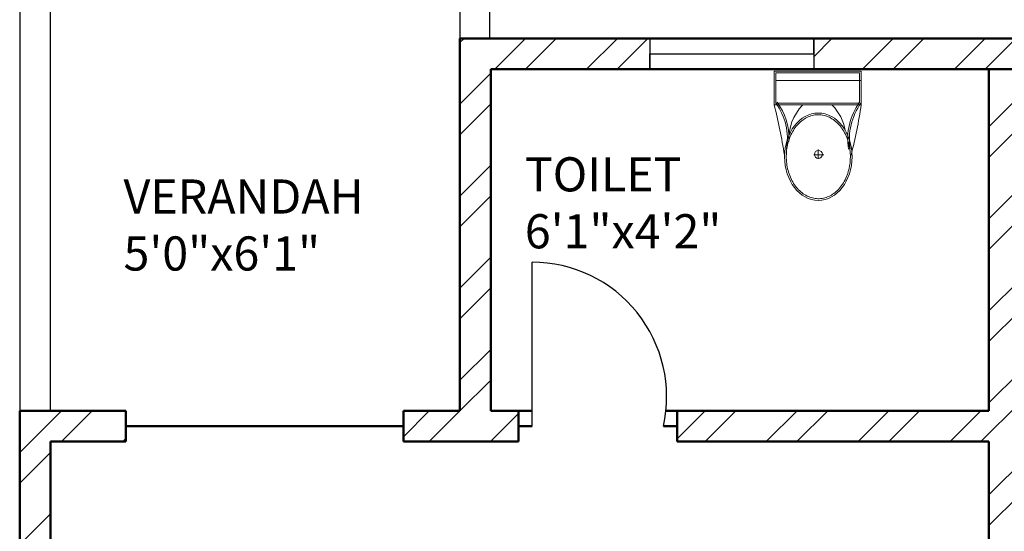
# Model space of a CAD drawing. Units: inches. Extents: x 1901 to 2863, y 888 to 2433.
# Tile 62 of 91: x 2025 to 2169, y 2202 to 2277. Entities that reach past the tile are written whole.
import ezdxf

# ---------------------------------------------------------------- set-up
doc = ezdxf.new("R2010")
doc.units = ezdxf.units.IN
for name, color, linetype, lineweight in [('A-AREA-IDEN', 7, 'Continuous', 18), ('A-DOOR', 4, 'Continuous', 25), ('A-FLOR-FIXT', 9, 'Continuous', 18), ('A-FLOR-HRAL', 41, 'Continuous', 25), ('A-GLAZ', 3, 'Continuous', 25), ('A-WALL', 7, 'Continuous', 50), ('A-WALL-PATT', 8, 'Continuous', 13)]:
    doc.layers.add(name, color=color, linetype=linetype, lineweight=lineweight)
doc.styles.get("Standard").update_dxf_attribs({"font": 'arial.ttf'})

# ---------------------------------------------------------------- blocks, each defined once
blk = doc.blocks.new('A$C31115884')
for p, q in [((283.1, 497.7), (223.4, 497.7)), ((257.5, 466.4), (257.5, 523.2)), ((0, 200), (0, 0)), ((520, 200), (0, 200)), ((10, 190), (10, 10)), ((510, 190), (10, 190)), ((510, 10), (510, 190)), ((520, 0), (520, 200)), ((510, 54.5), (0, 54.5)), ((10, 10), (510, 10)), ((0, 0), (520, 0))]:
    blk.add_line(p, q)
blk.add_circle((255.6, 496.4), 23.6)
for centre, radius, start, end in [((2777.7, -204.6), 2807, 165.4549, 171.71327), ((3237, 905), 2807, 188.28673, 194.5451), ((-294.5, 403.3), 364.7, 324.20913, 9.34987), ((-294.5, 403.3), 374.7, 324.20913, 9.34987), ((139.5, 406.2), 293.5, 315.84364, 2.65635), ((805.8, 403.3), 364.7, 170.65013, 215.79087), ((383.6, 406.2), 293.5, 190.27735, 224.15636), ((805.8, 403.3), 374.7, 179.20365, 215.79087)]:
    blk.add_arc(centre, radius, start, end)
blk.add_ellipse((256.2, 509.9), major_axis=(0, -260.7), ratio=0.772727)
blk.add_open_spline([(256.2, 259.2), (263.1, 259.2), (270, 259.7), (287.8, 262.3), (298.7, 265.1), (319.9, 273.1), (330.2, 278.4), (350.1, 291.1), (359.7, 298.7), (377.7, 315.9), (386.2, 325.5), (401.7, 346.6), (408.8, 358.1), (421.3, 382.5), (426.8, 395.5), (435.9, 422.4), (439.5, 436.4), (444.8, 465.1), (446.5, 479.7), (447.9, 509.2), (447.6, 524), (445, 553.3), (442.7, 567.8), (436.3, 596), (432.1, 609.7), (421.9, 636), (416, 648.6), (402.5, 672.1), (395, 683), (378.6, 703), (369.8, 712.1), (351.1, 728), (341.3, 734.8), (320.9, 746.2), (310.4, 750.7), (288.9, 757.3), (278, 759.4), (256, 761), (245, 760.6), (223.1, 757.2), (212.3, 754.3), (191.1, 746.1), (180.8, 740.7), (160.9, 727.8), (151.4, 720.1), (133.5, 702.7), (125.1, 693), (109.6, 671.7), (102.6, 660.2), (90.2, 635.7), (84.9, 622.7), (76, 595.6), (72.4, 581.6), (67.2, 552.9), (65.6, 538.2), (64.4, 508.8), (64.8, 494), (67.5, 464.7), (69.9, 450.2), (76.6, 422), (80.8, 408.3), (91.1, 382.2), (97.2, 369.7), (110.8, 346.3), (118.4, 335.4), (134.8, 315.6), (143.7, 306.7), (162.4, 290.9), (172.3, 284.2), (192.8, 273), (203.3, 268.6), (224.8, 262.2), (235.8, 260.2), (249.9, 259.3), (253, 259.2), (256.2, 259.2)], degree=3, knots=[0, 0, 0, 0, 0.110105, 0.110105, 0.285049, 0.285049, 0.459994, 0.459994, 0.634938, 0.634938, 0.809882, 0.809882, 0.984827, 0.984827, 1.159771, 1.159771, 1.334715, 1.334715, 1.50966, 1.50966, 1.684604, 1.684604, 1.859549, 1.859549, 2.034493, 2.034493, 2.209437, 2.209437, 2.384382, 2.384382, 2.559326, 2.559326, 2.73427, 2.73427, 2.909215, 2.909215, 3.084159, 3.084159, 3.259103, 3.259103, 3.434048, 3.434048, 3.608992, 3.608992, 3.783936, 3.783936, 3.958881, 3.958881, 4.133825, 4.133825, 4.30877, 4.30877, 4.483714, 4.483714, 4.658658, 4.658658, 4.833603, 4.833603, 5.008547, 5.008547, 5.183491, 5.183491, 5.358436, 5.358436, 5.53338, 5.53338, 5.708324, 5.708324, 5.883269, 5.883269, 6.058213, 6.058213, 6.233158, 6.233158, 6.283185, 6.283185, 6.283185, 6.283185])
blk = doc.blocks.new('WIN-24')
for p, q in [((0, 4.5), (0, 0)), ((24, 2.25), (24, 4.5)), ((24, 4.5), (24, 0)), ((0, 0), (0, 2.25)), ((0, 2.25), (24, 2.25))]:
    blk.add_line(p, q)
blk = doc.blocks.new('DOOR-20')
blk.add_line((0, -0.02), (0, 23.98))
blk.add_arc((0, 4.28), 19.71, 347.419, 90)

msp = doc.modelspace()

# ---------------------------------------------------------------- hatches: boundary and pattern name
at = {"layer": 'A-WALL-PATT'}
h = msp.add_hatch(dxfattribs=at)
h.set_pattern_fill('ANSI32', color=256)
h.paths.add_polyline_path([(2192.5, 2274.13), (2141.26, 2274.13), (2141.26, 2269.63), (2192.5, 2269.63)])
h.paths.add_polyline_path([(2259.93, 2274.13), (2216.5, 2274.13), (2216.5, 2269.63), (2255.43, 2269.63), (2255.43, 2214.63), (2250.81, 2214.63), (2250.81, 2210.13), (2259.93, 2210.13), (2259.93, 2215.13), (2271.76, 2215.13), (2271.76, 2217.38), (2271.76, 2219.63), (2259.93, 2219.63)])
h.paths.add_polyline_path([(2171.43, 2269.63), (2166.93, 2269.63), (2166.93, 2219.63), (2121.24, 2219.63), (2121.24, 2215.13), (2166.93, 2215.13), (2166.93, 2083.13), (2161.81, 2083.13), (2161.81, 2078.63), (2171.43, 2078.63), (2177, 2078.63), (2177, 2080.88), (2177, 2083.13), (2171.43, 2083.13), (2171.43, 2210.13), (2230.91, 2210.13), (2230.91, 2212.38), (2230.91, 2214.63), (2171.43, 2214.63)])
h.paths.add_polyline_path([(2117.26, 2274.13), (2089.43, 2274.13), (2089.43, 2219.63), (2081.14, 2219.63), (2081.14, 2215.13), (2089.43, 2215.13), (2098, 2215.13), (2098, 2217.38), (2098, 2219.63), (2093.93, 2219.63), (2093.93, 2269.63), (2117.26, 2269.63), (2117.26, 2271.88)])
h.paths.add_polyline_path([(2343.43, 2219.63), (2329.29, 2219.63), (2329.29, 2215.13), (2338.93, 2215.13), (2338.93, 2184.74), (2343.43, 2184.74)])
h.paths.add_polyline_path([(2338.93, 2083.13), (2329.29, 2083.13), (2208.97, 2083.13), (2208.97, 2078.63), (2338.93, 2078.63)])
h.paths.add_polyline_path([(2343.43, 2136.74), (2338.93, 2136.74), (2338.93, 1872.63), (2343.43, 1872.63)])
h.paths.add_polyline_path([(2343.43, 1863.63), (2397.68, 1863.63), (2397.68, 1821.63), (2384.14, 1821.63), (2384.14, 1812.63), (2418.33, 1812.63), (2418.33, 1817.13), (2418.33, 1821.63), (2406.68, 1821.63), (2406.68, 1863.63), (2459.5, 1863.63), (2459.5, 1821.63), (2447.14, 1821.63), (2447.14, 1812.63), (2459.5, 1812.63), (2468.5, 1812.63), (2468.5, 1872.63), (2394.43, 1872.63), (2334.43, 1872.63), (2334.43, 1812.63), (2343.43, 1812.63), (2353.25, 1812.63), (2353.25, 1821.63), (2343.43, 1821.63)])
h.paths.add_polyline_path([(2510.01, 1872.63), (2468.5, 1872.63), (2468.5, 1868.13), (2510.01, 1868.13)])
h.paths.add_polyline_path([(2514.01, 1817.13), (2468.5, 1817.13), (2468.5, 1812.63), (2482.11, 1812.63), (2482.11, 1800.61), (2486.61, 1800.61), (2486.61, 1812.63), (2514.01, 1812.63)])
h.paths.add_polyline_path([(2299.25, 1814.88), (2299.25, 1817.13), (2295.93, 1817.13), (2295.93, 1854.17), (2293.68, 1854.17), (2291.43, 1854.17), (2291.43, 1817.13), (2266.11, 1817.13), (2266.11, 1812.63), (2299.25, 1812.63)])
h.paths.add_polyline_path([(2218.11, 1817.13), (2206.46, 1817.13), (2171.43, 1817.13), (2171.43, 1949.13), (2190.1, 1949.13), (2190.1, 1953.63), (2163.47, 1953.63), (2163.47, 1949.13), (2166.93, 1949.13), (2166.93, 1817.13), (2114.3, 1817.13), (2114.3, 1812.63), (2218.11, 1812.63)])
h.paths.add_polyline_path([(2029.43, 1970.92), (2024.93, 1970.92), (2024.93, 1912.72), (2029.43, 1912.72)])
h.paths.add_polyline_path([(2132.3, 1953.63), (2113.93, 1953.63), (2113.93, 1975.89), (2111.68, 1975.89), (2109.43, 1975.89), (2109.43, 1953.63), (2029.43, 1953.63), (2029.43, 1949.13), (2132.3, 1949.13)])
h.paths.add_polyline_path([(2029.43, 1853.61), (2029.31, 1853.61), (2029.31, 1853.61), (2029.43, 1853.61), (2029.43, 1864.72), (2024.93, 1864.72), (2024.93, 1812.63), (2066.3, 1812.63), (2066.3, 1814.88), (2066.3, 1817.13), (2029.43, 1817.13)])
h.paths.add_polyline_path([(2122.93, 2010.09), (2120.68, 2010.09), (2118.43, 2010.09), (2118.43, 2006.13), (2029.43, 2006.13), (2029.43, 2001.63), (2109.43, 2001.63), (2109.43, 1998.04), (2113.93, 1998.04), (2113.93, 2001.63), (2122.93, 2001.63)])
h.paths.add_polyline_path([(2029.43, 2031.38), (2024.93, 2031.38), (2024.93, 1994.92), (2027.18, 1994.92), (2029.43, 1994.92)])
h.paths.add_polyline_path([(2029.43, 2136.74), (2024.93, 2136.74), (2024.93, 2067.38), (2027.18, 2067.38), (2029.43, 2067.38)])
h.paths.add_polyline_path([(2125.62, 2083.13), (2029.43, 2083.13), (2029.43, 2078.63), (2118.43, 2078.63), (2118.43, 2030.71), (2122.93, 2030.71), (2122.93, 2078.63), (2125.62, 2078.63)])
h.paths.add_polyline_path([(2029.43, 2215.13), (2040.47, 2215.13), (2040.47, 2217.38), (2040.47, 2219.63), (2024.93, 2219.63), (2024.93, 2184.74), (2029.43, 2184.74), (2029.43, 2187.78)])
h.paths.add_polyline_path([(2686.43, 2274.13), (2659.28, 2274.13), (2659.28, 2269.63), (2681.93, 2269.63), (2681.93, 2219.63), (2676.82, 2219.63), (2676.82, 2215.13), (2681.93, 2215.13), (2697.01, 2215.13), (2697.01, 2217.38), (2697.01, 2219.63), (2686.43, 2219.63)])
h.paths.add_polyline_path([(2609.93, 2269.63), (2635.28, 2269.63), (2635.28, 2274.13), (2571.43, 2274.13), (2571.43, 2269.63), (2605.43, 2269.63), (2605.43, 2214.63), (2549.1, 2214.63), (2549.1, 2210.13), (2605.43, 2210.13), (2605.43, 2083.13), (2601.01, 2083.13), (2601.01, 2080.88), (2601.01, 2078.63), (2609.93, 2078.63), (2616.16, 2078.63), (2616.16, 2080.88), (2616.16, 2083.13), (2609.93, 2083.13), (2609.93, 2215.13), (2651.46, 2215.13), (2651.46, 2217.38), (2651.46, 2219.63), (2609.93, 2219.63)])
h.paths.add_polyline_path([(2521.43, 2269.63), (2547.43, 2269.63), (2547.43, 2271.88), (2547.43, 2274.13), (2516.93, 2274.13), (2516.93, 2219.63), (2506.41, 2219.63), (2506.41, 2215.13), (2516.93, 2215.13), (2516.93, 2210.13), (2525.4, 2210.13), (2525.4, 2212.38), (2525.4, 2214.63), (2521.43, 2214.63)])
h.paths.add_polyline_path([(2456.01, 2219.63), (2439.43, 2219.63), (2439.43, 2187.89), (2443.93, 2187.89), (2443.93, 2215.13), (2456.01, 2215.13)])
h.paths.add_polyline_path([(2752.93, 2219.63), (2739.48, 2219.63), (2739.48, 2215.13), (2748.43, 2215.13), (2748.43, 2187.89), (2752.93, 2187.89)])
h.paths.add_polyline_path([(2752.93, 2139.89), (2748.43, 2139.89), (2748.43, 2083.13), (2648.42, 2083.13), (2648.42, 2078.63), (2654.93, 2078.63), (2654.93, 2039.44), (2659.43, 2039.44), (2659.43, 2078.63), (2748.43, 2078.63), (2748.43, 2063.43), (2752.93, 2063.43)])
h.paths.add_polyline_path([(2752.93, 2010.63), (2659.43, 2010.63), (2659.43, 2015.65), (2654.93, 2015.65), (2654.93, 2010.63), (2605.43, 2010.63), (2605.43, 1920.97), (2609.93, 1920.97), (2609.93, 2006.13), (2748.43, 2006.13), (2748.43, 1982.47), (2752.93, 1982.47)])
h.paths.add_polyline_path([(2752.93, 2027.43), (2748.43, 2027.43), (2748.43, 2010.63), (2752.93, 2010.63)])
h.paths.add_polyline_path([(2748.43, 1886.13), (2609.93, 1886.13), (2609.93, 1889.72), (2605.43, 1889.72), (2605.43, 1861.26), (2609.93, 1861.26), (2609.93, 1881.63), (2748.43, 1881.63)])
h.paths.add_polyline_path([(2456.86, 2228.83), (2498.4, 2228.83), (2498.4, 2247.49), (2456.86, 2247.49)], flags=9)
h.paths.add_polyline_path([(2038.6, 2237.42), (2080.17, 2237.42), (2080.17, 2256.08), (2038.6, 2256.08)], flags=9)
h.paths.add_polyline_path([(2292.01, 1062.39), (2539.93, 1062.39), (2539.93, 1099.49), (2292.01, 1099.49)], flags=9)
h.paths.add_polyline_path([(2424.91, 1832.25), (2448.51, 1832.25), (2448.51, 1846.68), (2424.91, 1846.68)], flags=25)
h.paths.add_polyline_path([(2359.08, 1832.25), (2382.68, 1832.25), (2382.68, 1846.68), (2359.08, 1846.68)], flags=25)
h.paths.add_polyline_path([(2352.9, 1684.8), (2367.54, 1684.8), (2367.54, 1697.17), (2352.9, 1697.17)], flags=9)
h.paths.add_polyline_path([(2079.29, 1755.83), (2169.02, 1755.83), (2169.02, 1774.37), (2079.29, 1774.37)], flags=9)
h.paths.add_polyline_path([(2404.09, 1373.86), (2404.09, 1463.59), (2385.54, 1463.59), (2385.54, 1373.86)], flags=9)
h.paths.add_polyline_path([(2268.09, 2236.37), (2309.64, 2236.37), (2309.64, 2255.03), (2268.09, 2255.03)], flags=9)
h.paths.add_polyline_path([(2575.96, 1700.95), (2665.7, 1700.95), (2665.7, 1719.5), (2575.96, 1719.5)], flags=9)
h.paths.add_polyline_path([(2302.96, 1878.47), (2329.52, 1878.47), (2329.52, 1888.78), (2302.96, 1888.78)], flags=9)
h.paths.add_polyline_path([(2097.42, 2240.58), (2126.57, 2240.58), (2126.57, 2259.23), (2097.42, 2259.23)], flags=9)
h.paths.add_polyline_path([(2208.72, 2246.12), (2237.88, 2246.12), (2237.88, 2264.78), (2208.72, 2264.78)], flags=9)
h.paths.add_polyline_path([(2038.15, 1925.96), (2076.99, 1925.96), (2076.99, 1944.62), (2038.15, 1944.62)], flags=9)
h.paths.add_polyline_path([(2239.14, 1926.67), (2288.46, 1926.67), (2288.46, 1945.33), (2239.14, 1945.33)], flags=9)
h.paths.add_polyline_path([(2175.43, 2007.33), (2212.36, 2007.33), (2212.36, 2025.99), (2175.43, 2025.99)], flags=9)
h.paths.add_polyline_path([(2225.03, 2091.79), (2263.87, 2091.79), (2263.87, 2110.45), (2225.03, 2110.45)], flags=9)
h.paths.add_polyline_path([(2035.4, 2098.48), (2074.24, 2098.48), (2074.24, 2117.14), (2035.4, 2117.14)], flags=9)
h.paths.add_polyline_path([(2050.1, 2029.21), (2083.26, 2029.21), (2083.26, 2047.87), (2050.1, 2047.87)], flags=9)
h.paths.add_polyline_path([(2069.68, 1956.72), (2098.83, 1956.72), (2098.83, 1975.38), (2069.68, 1975.38)], flags=25)
h.paths.add_polyline_path([(2328.62, 1753.34), (2361.66, 1753.34), (2361.66, 1771.99), (2328.62, 1771.99)], flags=9)
h.paths.add_polyline_path([(2395.16, 2060.89), (2395.16, 2140.65), (2378.68, 2140.65), (2378.68, 2060.89)], flags=9)
h.paths.add_polyline_path([(2463.73, 2059.02), (2492.89, 2059.02), (2492.89, 2077.68), (2463.73, 2077.68)], flags=9)
h.paths.add_polyline_path([(2458.03, 2181.54), (2496.87, 2181.54), (2496.87, 2200.19), (2458.03, 2200.19)], flags=9)
h.paths.add_polyline_path([(2527.58, 2243.07), (2556.73, 2243.07), (2556.73, 2261.73), (2527.58, 2261.73)], flags=9)
h.paths.add_polyline_path([(2694.46, 2232.77), (2736.03, 2232.77), (2736.03, 2251.42), (2694.46, 2251.42)], flags=9)
h.paths.add_polyline_path([(2637.82, 2249.22), (2666.98, 2249.22), (2666.98, 2267.88), (2637.82, 2267.88)], flags=9)
h.paths.add_polyline_path([(2623.69, 2183.54), (2662.53, 2183.54), (2662.53, 2202.2), (2623.69, 2202.2)], flags=9)
h.paths.add_polyline_path([(2691.97, 2021.5), (2725.12, 2021.5), (2725.12, 2040.16), (2691.97, 2040.16)], flags=9)
h.paths.add_polyline_path([(2621.04, 1975.91), (2662.34, 1975.91), (2662.34, 1994.57), (2621.04, 1994.57)], flags=25)
h.paths.add_polyline_path([(2479.03, 1927.62), (2519.84, 1927.62), (2519.84, 1946.28), (2479.03, 1946.28)], flags=9)
h.paths.add_polyline_path([(2670.94, 1849.08), (2716.01, 1849.08), (2716.01, 1867.73), (2670.94, 1867.73)], flags=9)
h.paths.add_polyline_path([(2523.61, 1782.96), (2550.17, 1782.96), (2550.17, 1793.26), (2523.61, 1793.26)], flags=9)
h.paths.add_polyline_path([(2450.84, 1207.33), (2492.39, 1207.33), (2492.39, 1225.99), (2450.84, 1225.99)], flags=9)
h.paths.add_polyline_path([(2527.75, 1203.84), (2556.91, 1203.84), (2556.91, 1222.5), (2527.75, 1222.5)], flags=9)
h.paths.add_polyline_path([(2639.11, 1207.2), (2668.27, 1207.2), (2668.27, 1225.86), (2639.11, 1225.86)], flags=9)
h.paths.add_polyline_path([(2692.59, 1218.97), (2734.17, 1218.97), (2734.17, 1237.62), (2692.59, 1237.62)], flags=9)
h.paths.add_polyline_path([(2669.27, 1366.33), (2708.11, 1366.33), (2708.11, 1384.99), (2669.27, 1384.99)], flags=9)
h.paths.add_polyline_path([(2463.31, 1358.03), (2502.15, 1358.03), (2502.15, 1376.69), (2463.31, 1376.69)], flags=9)
h.paths.add_polyline_path([(2494.72, 1449.96), (2531.65, 1449.96), (2531.65, 1468.62), (2494.72, 1468.62)], flags=9)
h.paths.add_polyline_path([(2675.57, 1422.16), (2708.72, 1422.16), (2708.72, 1440.81), (2675.57, 1440.81)], flags=9)
h.paths.add_polyline_path([(2685.63, 1493.89), (2714.79, 1493.89), (2714.79, 1512.55), (2685.63, 1512.55)], flags=9)
h.paths.add_polyline_path([(2686.8, 1529.91), (2725.65, 1529.91), (2725.65, 1548.57), (2686.8, 1548.57)], flags=9)
h.paths.add_polyline_path([(2503.65, 1537.99), (2552.97, 1537.99), (2552.97, 1556.65), (2503.65, 1556.65)], flags=9)
h.paths.add_polyline_path([(2291.71, 1643.5), (2318.28, 1643.5), (2318.28, 1653.81), (2291.71, 1653.81)], flags=9)
h.paths.add_polyline_path([(2450.63, 1610.52), (2477.19, 1610.52), (2477.19, 1620.82), (2450.63, 1620.82)], flags=9)
h.paths.add_polyline_path([(2359.99, 1551.81), (2422.25, 1551.81), (2422.25, 1562.12), (2359.99, 1562.12)], flags=9)
h.paths.add_polyline_path([(2280.11, 1249.01), (2321.65, 1249.01), (2321.65, 1267.66), (2280.11, 1267.66)], flags=9)
h.paths.add_polyline_path([(2164.06, 1274.23), (2193.22, 1274.23), (2193.22, 1292.89), (2164.06, 1292.89)], flags=9)
h.paths.add_polyline_path([(2118.21, 1277.69), (2151.25, 1277.69), (2151.25, 1296.35), (2118.21, 1296.35)], flags=9)
h.paths.add_polyline_path([(2031.95, 1268.53), (2073.52, 1268.53), (2073.52, 1287.19), (2031.95, 1287.19)], flags=9)
h.paths.add_polyline_path([(2050.2, 1409.08), (2089.04, 1409.08), (2089.04, 1427.74), (2050.2, 1427.74)], flags=9)
h.paths.add_polyline_path([(2243.74, 1421.03), (2282.58, 1421.03), (2282.58, 1439.69), (2243.74, 1439.69)], flags=9)
h.paths.add_polyline_path([(2190.75, 1509.77), (2231.56, 1509.77), (2231.56, 1528.43), (2190.75, 1528.43)], flags=9)
h.paths.add_polyline_path([(2058.39, 1475.42), (2091.55, 1475.42), (2091.55, 1494.07), (2058.39, 1494.07)], flags=9)
h.paths.add_polyline_path([(2062.45, 1553.09), (2091.6, 1553.09), (2091.6, 1571.75), (2062.45, 1571.75)], flags=9)
h.paths.add_polyline_path([(2219.52, 1590.37), (2266.15, 1590.37), (2266.15, 1609.02), (2219.52, 1609.02)], flags=9)
h.paths.add_polyline_path([(2041.07, 1584.19), (2079.91, 1584.19), (2079.91, 1602.85), (2041.07, 1602.85)], flags=9)
h = msp.add_hatch(dxfattribs=at)
h.set_pattern_fill('ANSI32', color=256)
h.paths.add_polyline_path([(2443.93, 2139.89), (2439.43, 2139.89), (2439.43, 2069.35), (2441.68, 2069.35), (2443.93, 2069.35), (2443.93, 2078.63), (2521.93, 2078.63), (2521.93, 2075.07), (2524.18, 2075.07), (2526.43, 2075.07), (2526.43, 2078.63), (2571.75, 2078.63), (2571.75, 2080.88), (2571.75, 2083.13), (2443.93, 2083.13)])
h.paths.add_polyline_path([(2526.43, 2054.63), (2524.18, 2054.63), (2521.93, 2054.63), (2521.93, 2030.63), (2443.93, 2030.63), (2443.93, 2045.35), (2439.43, 2045.35), (2439.43, 1983.87), (2443.93, 1983.87), (2443.93, 2026.13), (2521.93, 2026.13), (2526.43, 2026.13)])
h.paths.add_polyline_path([(2443.93, 1923.87), (2439.43, 1923.87), (2439.43, 1872.63), (2443.93, 1872.63)])
h.paths.add_polyline_path([(2636.23, 1766.13), (2609.93, 1766.13), (2609.93, 1779.79), (2605.43, 1779.79), (2605.43, 1766.13), (2486.61, 1766.13), (2486.61, 1770.67), (2482.11, 1770.67), (2482.11, 1766.13), (2482.11, 1761.63), (2636.23, 1761.63), (2636.23, 1763.88)])
h.paths.add_polyline_path([(2519.54, 1663.38), (2519.54, 1665.63), (2494.93, 1665.63), (2481.83, 1665.63), (2481.83, 1663.38), (2481.83, 1661.13), (2490.43, 1661.13), (2490.43, 1640.16), (2494.93, 1640.16), (2494.93, 1661.13), (2519.54, 1661.13)])
h.paths.add_polyline_path([(2443.93, 1712.13), (2443.93, 1716.63), (2414.46, 1716.63), (2414.46, 1712.13), (2439.43, 1712.13), (2439.43, 1545.51), (2443.93, 1545.51), (2443.93, 1661.13), (2448.47, 1661.13), (2448.47, 1665.63), (2443.93, 1665.63)])
h.paths.add_polyline_path([(2343.43, 1712.13), (2365.52, 1712.13), (2365.52, 1714.38), (2365.52, 1716.63), (2333.87, 1716.63), (2333.87, 1714.38), (2333.87, 1712.13), (2338.93, 1712.13), (2338.93, 1575.63), (2338.93, 1545.51), (2343.43, 1545.51), (2343.43, 1547.51), (2343.43, 1580.13)])
h.paths.add_polyline_path([(2752.93, 1665.63), (2579.54, 1665.63), (2579.54, 1661.13), (2615.93, 1661.13), (2615.93, 1529.13), (2598.93, 1529.13), (2598.93, 1524.63), (2623.13, 1524.63), (2623.13, 1526.88), (2623.13, 1529.13), (2620.43, 1529.13), (2620.43, 1661.13), (2748.43, 1661.13), (2748.43, 1633.5), (2752.93, 1633.5)])
h.paths.add_polyline_path([(2752.93, 1419.93), (2748.43, 1419.93), (2748.43, 1400.13), (2659.43, 1400.13), (2659.43, 1444.33), (2657.18, 1444.33), (2654.93, 1444.33), (2654.93, 1400.13), (2643.65, 1400.13), (2643.65, 1395.63), (2748.43, 1395.63), (2748.43, 1364.04), (2752.93, 1364.04)])
h.paths.add_polyline_path([(2752.93, 1492.88), (2748.43, 1492.88), (2748.43, 1476.63), (2667.43, 1476.63), (2667.43, 1479.71), (2665.18, 1479.71), (2662.93, 1479.71), (2662.93, 1476.63), (2654.93, 1476.63), (2654.93, 1469.54), (2659.43, 1469.54), (2659.43, 1472.13), (2748.43, 1472.13), (2748.43, 1455.93), (2752.93, 1455.93)])
h.paths.add_polyline_path([(2752.93, 1304.04), (2748.43, 1304.04), (2748.43, 1263.63), (2738.66, 1263.63), (2738.66, 1259.13), (2752.93, 1259.13)])
h.paths.add_polyline_path([(2685.93, 1259.13), (2695.49, 1259.13), (2695.49, 1261.38), (2695.49, 1263.63), (2677.84, 1263.63), (2677.84, 1261.38), (2677.84, 1259.13), (2681.43, 1259.13), (2681.43, 1203.63), (2653.28, 1203.63), (2653.28, 1199.13), (2685.93, 1199.13), (2685.93, 1203.63)])
h.paths.add_polyline_path([(2609.43, 1395.63), (2611.85, 1395.63), (2611.85, 1400.13), (2598.89, 1400.13), (2598.89, 1397.88), (2598.89, 1395.63), (2604.93, 1395.63), (2604.93, 1268.13), (2554.73, 1268.13), (2554.73, 1265.88), (2554.73, 1263.63), (2604.93, 1263.63), (2604.93, 1203.63), (2571.31, 1203.63), (2571.31, 1199.13), (2604.93, 1199.13), (2629.28, 1199.13), (2629.28, 1201.38), (2629.28, 1203.63), (2609.43, 1203.63), (2609.43, 1258.63), (2609.43, 1259.13), (2654.8, 1259.13), (2654.8, 1263.63), (2609.43, 1263.63)])
h.paths.add_polyline_path([(2443.93, 1304.04), (2439.43, 1304.04), (2439.43, 1259.13), (2443.93, 1259.13), (2456.16, 1259.13), (2456.16, 1261.38), (2456.16, 1263.63), (2443.93, 1263.63)])
h.paths.add_polyline_path([(2525.43, 1263.63), (2531.78, 1263.63), (2531.78, 1268.13), (2520.93, 1268.13), (2520.93, 1263.63), (2511.41, 1263.63), (2511.41, 1259.13), (2520.93, 1259.13), (2520.93, 1199.13), (2547.31, 1199.13), (2547.31, 1201.38), (2547.31, 1203.63), (2525.43, 1203.63)])
h.paths.add_polyline_path([(2443.93, 1434.84), (2439.43, 1434.84), (2439.43, 1364.04), (2441.68, 1364.04), (2443.93, 1364.04)])
h.paths.add_polyline_path([(2567.13, 1400.13), (2443.93, 1400.13), (2443.93, 1395.63), (2567.13, 1395.63)])
h.paths.add_polyline_path([(2443.93, 1545.51), (2439.43, 1545.51), (2439.43, 1494.84), (2443.93, 1494.84)])
h.paths.add_polyline_path([(2494.93, 1553.35), (2492.68, 1553.35), (2490.43, 1553.35), (2490.43, 1524.63), (2494.93, 1524.63), (2525.94, 1524.63), (2525.94, 1526.88), (2525.94, 1529.13), (2494.93, 1529.13)])
h.paths.add_polyline_path([(2752.93, 1573.5), (2748.43, 1573.5), (2748.43, 1529.13), (2657.76, 1529.13), (2657.76, 1524.63), (2662.93, 1524.63), (2662.93, 1498.63), (2667.43, 1498.63), (2667.43, 1524.63), (2748.43, 1524.63), (2748.43, 1516.88), (2752.93, 1516.88)])
h.paths.add_polyline_path([(2038.6, 2237.42), (2080.17, 2237.42), (2080.17, 2256.08), (2038.6, 2256.08)], flags=9)
h.paths.add_polyline_path([(2292.01, 1062.39), (2539.93, 1062.39), (2539.93, 1099.49), (2292.01, 1099.49)], flags=9)
h.paths.add_polyline_path([(2424.91, 1832.25), (2448.51, 1832.25), (2448.51, 1846.68), (2424.91, 1846.68)], flags=9)
h.paths.add_polyline_path([(2359.08, 1832.25), (2382.68, 1832.25), (2382.68, 1846.68), (2359.08, 1846.68)], flags=9)
h.paths.add_polyline_path([(2352.9, 1684.8), (2367.54, 1684.8), (2367.54, 1697.17), (2352.9, 1697.17)], flags=9)
h.paths.add_polyline_path([(2079.29, 1755.83), (2169.02, 1755.83), (2169.02, 1774.37), (2079.29, 1774.37)], flags=9)
h.paths.add_polyline_path([(2404.09, 1373.86), (2404.09, 1463.59), (2385.54, 1463.59), (2385.54, 1373.86)], flags=9)
h.paths.add_polyline_path([(2268.09, 2236.37), (2309.64, 2236.37), (2309.64, 2255.03), (2268.09, 2255.03)], flags=9)
h.paths.add_polyline_path([(2575.96, 1700.95), (2665.7, 1700.95), (2665.7, 1719.5), (2575.96, 1719.5)], flags=9)
h.paths.add_polyline_path([(2302.96, 1878.47), (2329.52, 1878.47), (2329.52, 1888.78), (2302.96, 1888.78)], flags=9)
h.paths.add_polyline_path([(2097.42, 2240.58), (2126.57, 2240.58), (2126.57, 2259.23), (2097.42, 2259.23)], flags=9)
h.paths.add_polyline_path([(2208.72, 2246.12), (2237.88, 2246.12), (2237.88, 2264.78), (2208.72, 2264.78)], flags=9)
h.paths.add_polyline_path([(2038.15, 1925.96), (2076.99, 1925.96), (2076.99, 1944.62), (2038.15, 1944.62)], flags=9)
h.paths.add_polyline_path([(2239.14, 1926.67), (2288.46, 1926.67), (2288.46, 1945.33), (2239.14, 1945.33)], flags=9)
h.paths.add_polyline_path([(2175.43, 2007.33), (2212.36, 2007.33), (2212.36, 2025.99), (2175.43, 2025.99)], flags=9)
h.paths.add_polyline_path([(2225.03, 2091.79), (2263.87, 2091.79), (2263.87, 2110.45), (2225.03, 2110.45)], flags=9)
h.paths.add_polyline_path([(2035.4, 2098.48), (2074.24, 2098.48), (2074.24, 2117.14), (2035.4, 2117.14)], flags=9)
h.paths.add_polyline_path([(2050.1, 2029.21), (2083.26, 2029.21), (2083.26, 2047.87), (2050.1, 2047.87)], flags=9)
h.paths.add_polyline_path([(2069.68, 1956.72), (2098.83, 1956.72), (2098.83, 1975.38), (2069.68, 1975.38)], flags=9)
h.paths.add_polyline_path([(2328.62, 1753.34), (2361.66, 1753.34), (2361.66, 1771.99), (2328.62, 1771.99)], flags=9)
h.paths.add_polyline_path([(2395.16, 2060.89), (2395.16, 2140.65), (2378.68, 2140.65), (2378.68, 2060.89)], flags=9)
h.paths.add_polyline_path([(2463.73, 2059.02), (2492.89, 2059.02), (2492.89, 2077.68), (2463.73, 2077.68)], flags=9)
h.paths.add_polyline_path([(2458.03, 2181.54), (2496.87, 2181.54), (2496.87, 2200.19), (2458.03, 2200.19)], flags=9)
h.paths.add_polyline_path([(2456.86, 2228.83), (2498.4, 2228.83), (2498.4, 2247.49), (2456.86, 2247.49)], flags=9)
h.paths.add_polyline_path([(2527.58, 2243.07), (2556.73, 2243.07), (2556.73, 2261.73), (2527.58, 2261.73)], flags=9)
h.paths.add_polyline_path([(2694.46, 2232.77), (2736.03, 2232.77), (2736.03, 2251.42), (2694.46, 2251.42)], flags=9)
h.paths.add_polyline_path([(2637.82, 2249.22), (2666.98, 2249.22), (2666.98, 2267.88), (2637.82, 2267.88)], flags=9)
h.paths.add_polyline_path([(2623.69, 2183.54), (2662.53, 2183.54), (2662.53, 2202.2), (2623.69, 2202.2)], flags=9)
h.paths.add_polyline_path([(2691.97, 2021.5), (2725.12, 2021.5), (2725.12, 2040.16), (2691.97, 2040.16)], flags=9)
h.paths.add_polyline_path([(2621.04, 1975.91), (2662.34, 1975.91), (2662.34, 1994.57), (2621.04, 1994.57)], flags=9)
h.paths.add_polyline_path([(2479.03, 1927.62), (2519.84, 1927.62), (2519.84, 1946.28), (2479.03, 1946.28)], flags=9)
h.paths.add_polyline_path([(2670.94, 1849.08), (2716.01, 1849.08), (2716.01, 1867.73), (2670.94, 1867.73)], flags=9)
h.paths.add_polyline_path([(2523.61, 1782.96), (2550.17, 1782.96), (2550.17, 1793.26), (2523.61, 1793.26)], flags=9)
h.paths.add_polyline_path([(2450.84, 1207.33), (2492.39, 1207.33), (2492.39, 1225.99), (2450.84, 1225.99)], flags=9)
h.paths.add_polyline_path([(2527.75, 1203.84), (2556.91, 1203.84), (2556.91, 1222.5), (2527.75, 1222.5)], flags=9)
h.paths.add_polyline_path([(2639.11, 1207.2), (2668.27, 1207.2), (2668.27, 1225.86), (2639.11, 1225.86)], flags=9)
h.paths.add_polyline_path([(2692.59, 1218.97), (2734.17, 1218.97), (2734.17, 1237.62), (2692.59, 1237.62)], flags=9)
h.paths.add_polyline_path([(2669.27, 1366.33), (2708.11, 1366.33), (2708.11, 1384.99), (2669.27, 1384.99)], flags=25)
h.paths.add_polyline_path([(2463.31, 1358.03), (2502.15, 1358.03), (2502.15, 1376.69), (2463.31, 1376.69)], flags=9)
h.paths.add_polyline_path([(2494.72, 1449.96), (2531.65, 1449.96), (2531.65, 1468.62), (2494.72, 1468.62)], flags=9)
h.paths.add_polyline_path([(2675.57, 1422.16), (2708.72, 1422.16), (2708.72, 1440.81), (2675.57, 1440.81)], flags=25)
h.paths.add_polyline_path([(2685.63, 1493.89), (2714.79, 1493.89), (2714.79, 1512.55), (2685.63, 1512.55)], flags=9)
h.paths.add_polyline_path([(2686.8, 1529.91), (2725.65, 1529.91), (2725.65, 1548.57), (2686.8, 1548.57)], flags=25)
h.paths.add_polyline_path([(2503.65, 1537.99), (2552.97, 1537.99), (2552.97, 1556.65), (2503.65, 1556.65)], flags=9)
h.paths.add_polyline_path([(2291.71, 1643.5), (2318.28, 1643.5), (2318.28, 1653.81), (2291.71, 1653.81)], flags=9)
h.paths.add_polyline_path([(2450.63, 1610.52), (2477.19, 1610.52), (2477.19, 1620.82), (2450.63, 1620.82)], flags=9)
h.paths.add_polyline_path([(2359.99, 1551.81), (2422.25, 1551.81), (2422.25, 1562.12), (2359.99, 1562.12)], flags=9)
h.paths.add_polyline_path([(2280.11, 1249.01), (2321.65, 1249.01), (2321.65, 1267.66), (2280.11, 1267.66)], flags=9)
h.paths.add_polyline_path([(2164.06, 1274.23), (2193.22, 1274.23), (2193.22, 1292.89), (2164.06, 1292.89)], flags=9)
h.paths.add_polyline_path([(2118.21, 1277.69), (2151.25, 1277.69), (2151.25, 1296.35), (2118.21, 1296.35)], flags=9)
h.paths.add_polyline_path([(2031.95, 1268.53), (2073.52, 1268.53), (2073.52, 1287.19), (2031.95, 1287.19)], flags=9)
h.paths.add_polyline_path([(2050.2, 1409.08), (2089.04, 1409.08), (2089.04, 1427.74), (2050.2, 1427.74)], flags=9)
h.paths.add_polyline_path([(2243.74, 1421.03), (2282.58, 1421.03), (2282.58, 1439.69), (2243.74, 1439.69)], flags=9)
h.paths.add_polyline_path([(2190.75, 1509.77), (2231.56, 1509.77), (2231.56, 1528.43), (2190.75, 1528.43)], flags=9)
h.paths.add_polyline_path([(2058.39, 1475.42), (2091.55, 1475.42), (2091.55, 1494.07), (2058.39, 1494.07)], flags=9)
h.paths.add_polyline_path([(2062.45, 1553.09), (2091.6, 1553.09), (2091.6, 1571.75), (2062.45, 1571.75)], flags=9)
h.paths.add_polyline_path([(2219.52, 1590.37), (2266.15, 1590.37), (2266.15, 1609.02), (2219.52, 1609.02)], flags=9)
h.paths.add_polyline_path([(2041.07, 1584.19), (2079.91, 1584.19), (2079.91, 1602.85), (2041.07, 1602.85)], flags=9)

# ---------------------------------------------------------------- linework, layer by layer
at = {"layer": 'A-FLOR-HRAL'}
for p, q in [((2029.43, 2219.63), (2029.43, 2292.63)), ((2024.93, 2284.13), (2024.93, 2219.63)), ((2089.43, 2279.63), (2089.43, 2274.13)), ((2093.82, 2274.13), (2093.82, 2279.63))]:
    msp.add_line(p, q, dxfattribs=at)
at = {"layer": 'A-WALL'}
for p, q in [((2089.43, 2274.13), (2259.93, 2274.13)), ((2089.43, 2274.13), (2089.43, 2219.63)), ((2093.93, 2269.63), (2255.43, 2269.63)), ((2093.93, 2269.63), (2093.93, 2219.63)), ((2166.93, 2269.63), (2166.93, 2219.63)), ((2024.93, 2219.63), (2024.93, 1812.63)), ((2024.93, 2219.63), (2040.47, 2219.63)), ((2040.47, 2219.63), (2040.47, 2215.13)), ((2081.14, 2217.38), (2081.14, 2219.63)), ((2081.14, 2219.63), (2081.14, 2215.13)), ((2081.14, 2219.63), (2089.43, 2219.63)), ((2093.93, 2219.63), (2100, 2219.63)), ((2098, 2219.63), (2098, 2215.13)), ((2119.61, 2219.63), (2166.93, 2219.63)), ((2121.24, 2219.63), (2121.24, 2215.13)), ((2040.47, 2215.13), (2040.47, 2217.38)), ((2040.47, 2217.38), (2076.57, 2217.38)), ((2076.57, 2217.38), (2081.14, 2217.38)), ((2098, 2215.13), (2098, 2217.38)), ((2098, 2217.38), (2098, 2217.38)), ((2098, 2217.38), (2100, 2217.38)), ((2121.24, 2217.38), (2119.24, 2217.38)), ((2121.24, 2215.13), (2121.24, 2217.38)), ((2029.43, 2215.13), (2029.43, 1817.13)), ((2029.43, 2215.13), (2040.47, 2215.13)), ((2081.14, 2215.13), (2089.43, 2215.13)), ((2089.43, 2215.13), (2098, 2215.13)), ((2121.24, 2215.13), (2166.93, 2215.13)), ((2166.93, 2215.13), (2166.93, 2083.13))]:
    msp.add_line(p, q, dxfattribs=at)

# ---------------------------------------------------------------- block references
at = {"layer": 'A-DOOR'}
msp.add_blockref('DOOR-20', (2100, 2217.4), dxfattribs=at)
at = {"layer": 'A-FLOR-FIXT', "xscale": 0.0245149588751191, "yscale": 0.0245149588751191, "zscale": 0.0245149588751191, "rotation": 180}
msp.add_blockref('A$C31115884', (2148.21, 2269.33), dxfattribs=at)
at = {"layer": 'A-GLAZ'}
msp.add_blockref('WIN-24', (2117.26, 2269.63), dxfattribs=at)

# ---------------------------------------------------------------- texts
at = {"layer": 'A-AREA-IDEN', "char_height": 5, "attachment_point": 1}
for s, width, insert in [('TOILET\\P6\'1"x4\'2"', 67.9983, (2098.93, 2256.75)), ('VERANDAH\\P5\'0"x6\'1"', 131.2848, (2040.14, 2253.5))]:
    msp.add_mtext_dynamic_manual_height_columns(s, width=width, gutter_width=12.5, heights=[0], dxfattribs=dict(at, insert=insert))

doc.saveas('drawing.dxf')
